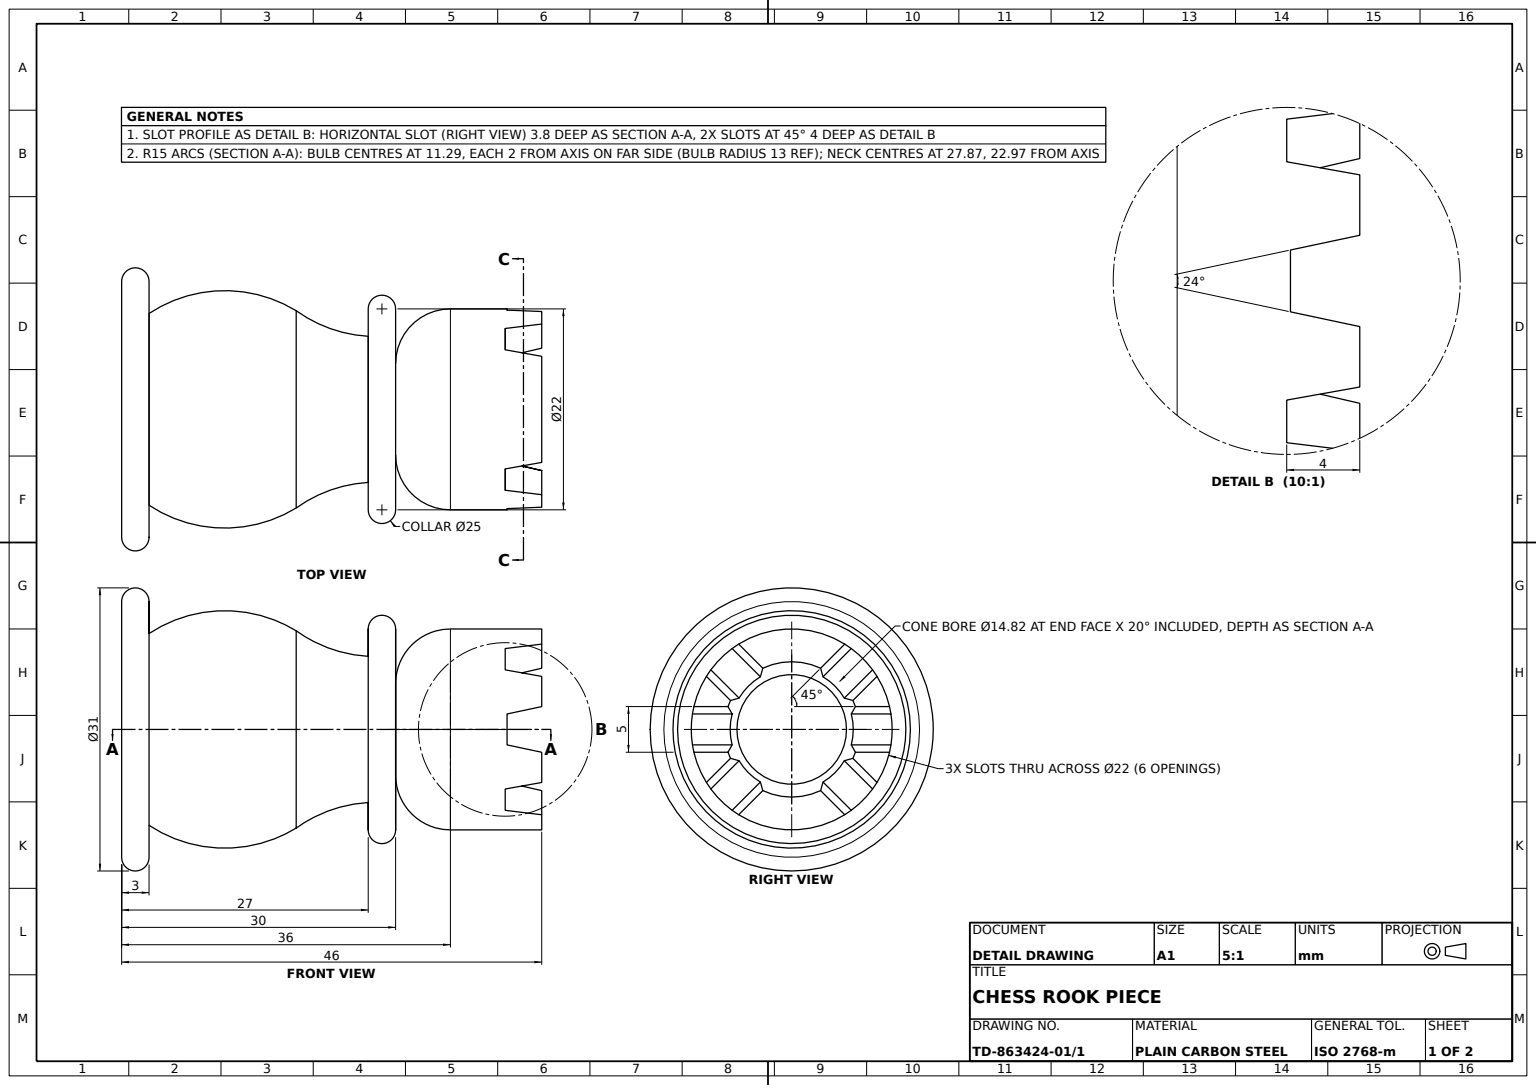
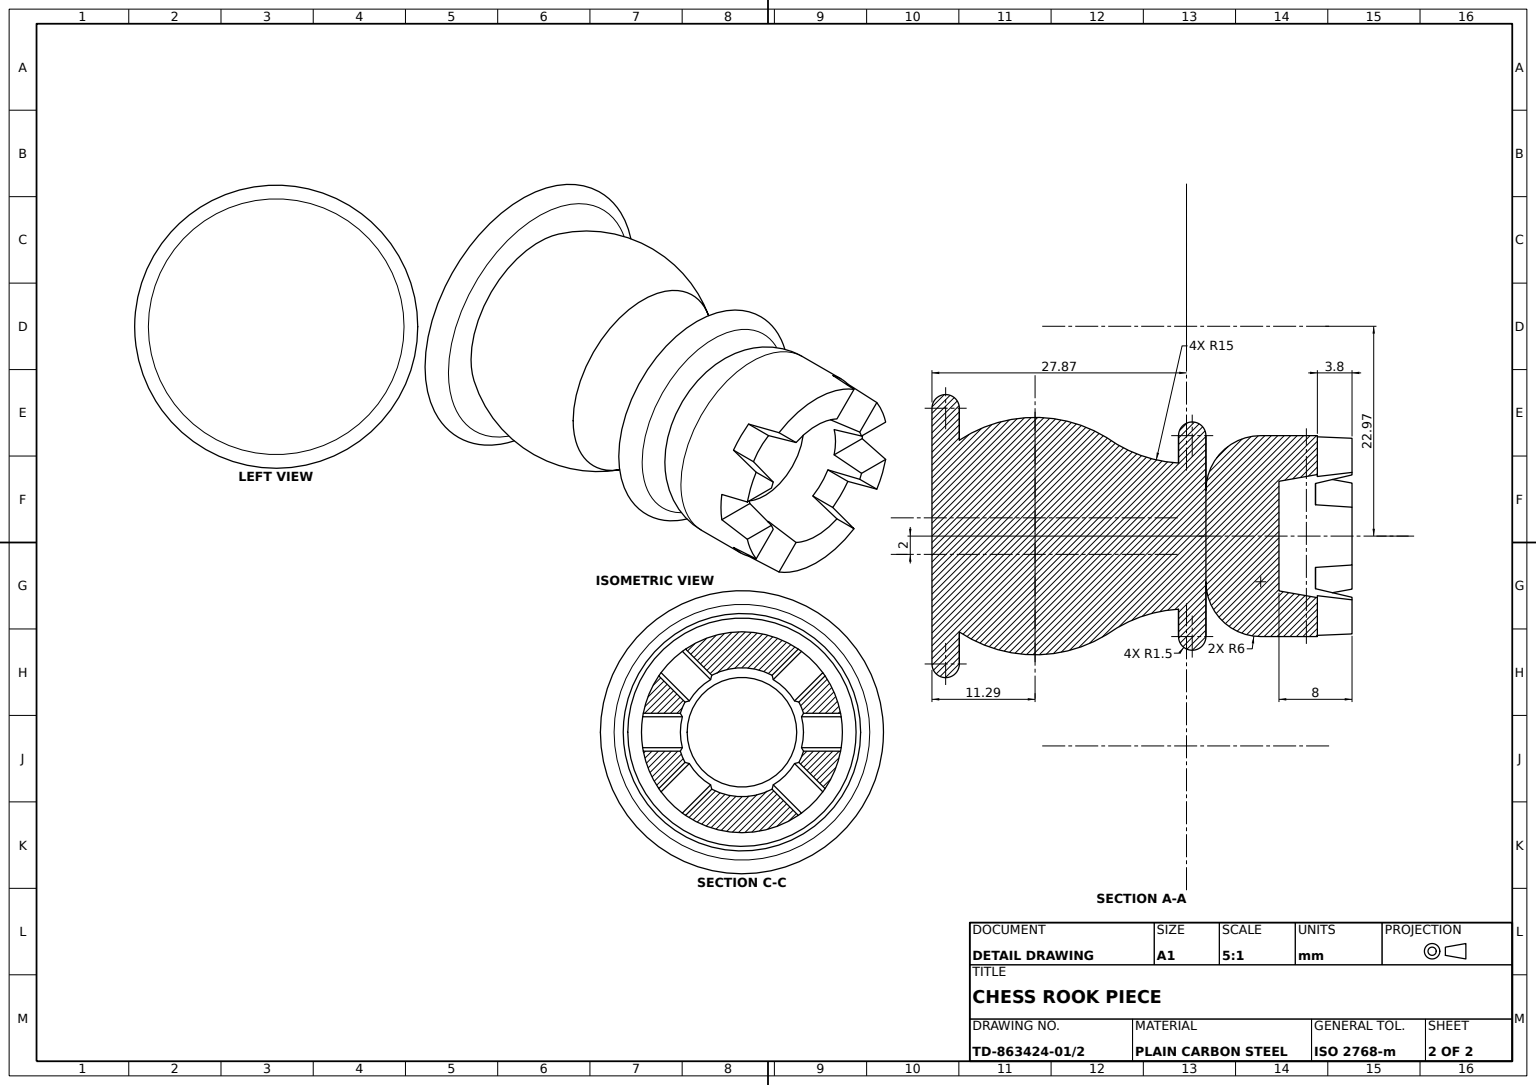
from build123d import *

# Parameters (mm, degrees)
CRENEL_SLOT_1_DEPTH = 35
CRENEL_SLOT_2_DEPTH = 35
CRENEL_SLOT_3_DEPTH = 35


with BuildPart() as part:
    # Rook Profile Sketch → Rook Body Revolve (revolve)
    with BuildSketch(Plane.XY, mode=Mode.PRIVATE) as rook_body_revolve_sk:
        with BuildLine():
            Line((-14, 0), (0, 0))
            Line((0, 0), (0, 11.291561976))
            Line((0, 11.291561976), (0, 46))
            Line((0, 46), (-11, 46))
            Line((-11, 46), (-11, 36))
            ThreePointArc((-11, 36), (-9.242640687, 31.757359313), (-5, 30))
            Line((-5, 30), (-11, 30))
            ThreePointArc((-11, 30), (-12.5, 28.5), (-11, 27))
            Line((-11, 27), (-8, 27))
            ThreePointArc((-8, 27), (-8.838560173, 22.857127729), (-10.799610921, 19.112684675))
            ThreePointArc((-10.799610921, 19.112684675), (-12.997407444, 11.012689327), (-10.5, 3))
            Line((-10.5, 3), (-14, 3))
            ThreePointArc((-14, 3), (-15.5, 1.5), (-14, 0))
        make_face()
    revolve(rook_body_revolve_sk.sketch.rotate(Axis((0, 0, 0), (0, 1, 0)), 270), axis=Axis((0, 0, 0), (0, 1, 0)))

    # Top Bore Sketch → Top Bore Cut (revolve, cut)
    with BuildSketch(Plane.XY, mode=Mode.PRIVATE) as top_bore_cut_sk:
        Polygon((0, 38), (-6, 38), (-7.410615846, 46), (0, 46), align=None)
    revolve(top_bore_cut_sk.sketch.rotate(Axis((0, 0, 0), (0, 1, 0)), 270), axis=Axis((0, 0, 0), (0, 1, 0)), mode=Mode.SUBTRACT)

    # Crenel Slot 1 Sketch → Crenel Slot 1 (cut, symmetric)
    with BuildSketch(Plane.XY):
        Polygon((-2.5, 46), (2.5, 46), (1.693128152, 42.203966408), (-1.693128152, 42.203966408), align=None)
    extrude(amount=CRENEL_SLOT_1_DEPTH, both=True, mode=Mode.SUBTRACT)

    # Crenel Slot 2 Sketch → Crenel Slot 2 (cut, symmetric)
    with BuildSketch(Plane(origin=(0, 0, 0), x_dir=(-0.7071067811865457, 0, 0.7071067811865493), z_dir=(0.7071067811865493, 0, 0.7071067811865457))):
        Polygon((-2.5, -46), (2.5, -46), (1.649773753, -42), (-1.649773753, -42), align=None)
    extrude(amount=CRENEL_SLOT_2_DEPTH, both=True, mode=Mode.SUBTRACT)

    # Crenel Slot 3 Sketch → Crenel Slot 3 (cut, symmetric)
    with BuildSketch(Plane(origin=(0, 0, 0), x_dir=(0.7071067811865465, 0, 0.7071067811865487), z_dir=(0.7071067811865487, 0, -0.7071067811865465))):
        Polygon((-2.5, -46), (2.5, -46), (1.649773753, -42), (-1.649773753, -42), align=None)
    extrude(amount=CRENEL_SLOT_3_DEPTH, both=True, mode=Mode.SUBTRACT)


solid = part.part
